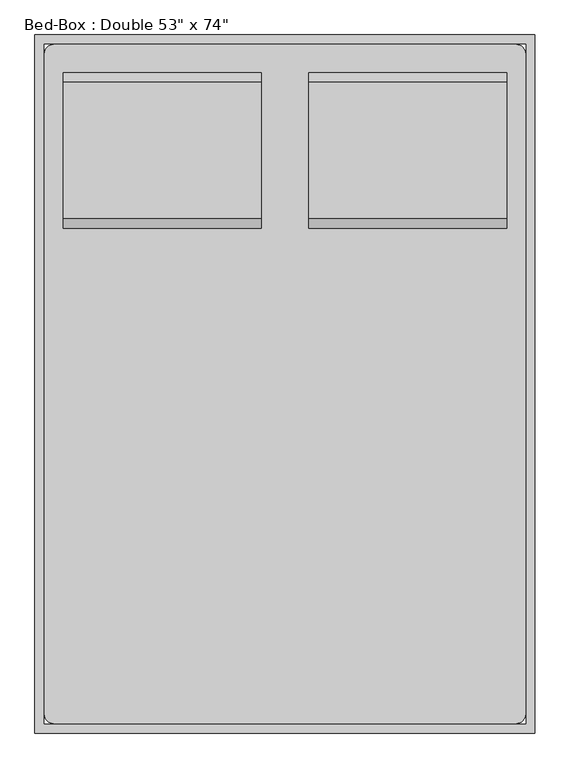
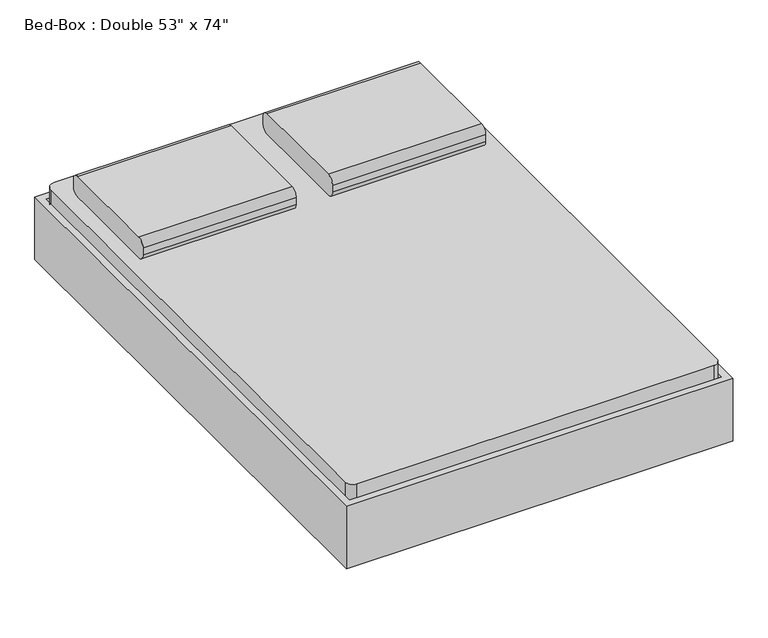
"""IFC4 building model written with IfcOpenShell, lengths in millimetres: furniture geometry."""

from ifc_helpers import new_model, si_unit, point, frame, frame_2d, origin, place, context, project, spatial, polyline, circle_curve, trimmed, segment, composite_curve, outline, extrude, source, transform, mapped, element, save
from ifc_brep_helpers import plane_surface, cylinder_surface, revolved_surface, advanced_brep


def furniture_c8abb964(model_context):
    return source(origin(), model_context, "Body", "SolidModel", [
        extrude(outline(composite_curve([segment(polyline([(578.3704918, 406.4), (210.0704918, 406.4)]), True, "CONTINUOUS"), segment(trimmed(circle_curve(frame_2d((210.0704918, 431.8)), 25.4), [point((210.0704918, 406.4))], [point((184.6704918, 431.8))], False, "CARTESIAN"), True, "CONTINUOUS"), segment(polyline([(184.6704918, 431.8), (184.6704918, 457.2)]), True, "CONTINUOUS"), segment(trimmed(circle_curve(frame_2d((210.0704918, 457.2)), 25.4), [point((184.6704918, 457.2))], [point((210.0704918, 482.6))], False, "CARTESIAN"), True, "CONTINUOUS"), segment(polyline([(210.0704918, 482.6), (578.3704918, 482.6)]), True, "CONTINUOUS"), segment(trimmed(circle_curve(frame_2d((578.3704918, 457.2)), 25.4), [point((578.3704918, 482.6))], [point((603.7704918, 457.2))], False, "CARTESIAN"), True, "CONTINUOUS"), segment(polyline([(603.7704918, 457.2), (603.7704918, 431.8)]), True, "CONTINUOUS"), segment(trimmed(circle_curve(frame_2d((578.3704918, 431.8)), 25.4), [point((603.7704918, 431.8))], [point((578.3704918, 406.4))], False, "CARTESIAN"), True, "CONTINUOUS")], self_intersect=False)), frame((402.652459, 0.0, 0.0), z_axis=(1.0, 0.0, 0.0), x_axis=(0.0, 1.0, 0.0)), (0.0, 0.0, 1.0), 533.4),
        extrude(outline(composite_curve([segment(polyline([(578.3704918, 406.4), (210.0704918, 406.4)]), True, "CONTINUOUS"), segment(trimmed(circle_curve(frame_2d((210.0704918, 431.8)), 25.4), [point((210.0704918, 406.4))], [point((184.6704918, 431.8))], False, "CARTESIAN"), True, "CONTINUOUS"), segment(polyline([(184.6704918, 431.8), (184.6704918, 457.2)]), True, "CONTINUOUS"), segment(trimmed(circle_curve(frame_2d((210.0704918, 457.2)), 25.4), [point((184.6704918, 457.2))], [point((210.0704918, 482.6))], False, "CARTESIAN"), True, "CONTINUOUS"), segment(polyline([(210.0704918, 482.6), (578.3704918, 482.6)]), True, "CONTINUOUS"), segment(trimmed(circle_curve(frame_2d((578.3704918, 457.2)), 25.4), [point((578.3704918, 482.6))], [point((603.7704918, 457.2))], False, "CARTESIAN"), True, "CONTINUOUS"), segment(polyline([(603.7704918, 457.2), (603.7704918, 431.8)]), True, "CONTINUOUS"), segment(trimmed(circle_curve(frame_2d((578.3704918, 431.8)), 25.4), [point((603.7704918, 431.8))], [point((578.3704918, 406.4))], False, "CARTESIAN"), True, "CONTINUOUS")], self_intersect=False)), frame((-257.747541, 0.0, 0.0), z_axis=(1.0, 0.0, 0.0), x_axis=(0.0, 1.0, 0.0)), (0.0, 0.0, 1.0), 533.4),
        advanced_brep(
        [(-308.2231784, 451.3704918, 177.8), (-308.2231784, 375.1704918, 177.8), (-308.2231784, 375.1704918, 196.85), (-308.2231784, 451.3704918, 196.85), (-257.4231784, 451.3704918, 177.8), (-257.4231784, 375.1704918, 177.8), (-245.2869899, 375.1704918, 196.85), (-245.2869899, 451.3704918, 196.85), (-181.3523099, 451.3704918, 14.6654962), (-181.3523099, 375.1704918, 14.6654962), (-164.0871466, 375.1704918, 22.716374), (-164.0871466, 451.3704918, 22.716374), (-158.3320921, 375.1704918, 0.0), (-158.3320921, 451.3704918, 0.0), (-158.3320921, 375.1704918, 19.05), (-158.3320921, 451.3704918, 19.05), (-79.7195862, 451.3704918, 0.0), (-79.7195862, 375.1704918, 0.0), (-79.7195862, 375.1704918, 19.05), (-79.7195862, 451.3704918, 19.05), (-67.0195862, 375.1704918, 3.4029547), (-67.0195862, 451.3704918, 3.4029547), (-76.5445862, 375.1704918, 19.9007387), (-76.5445862, 451.3704918, 19.9007387), (-6.922541, 451.3704918, 38.1), (-6.922541, 375.1704918, 38.1), (-12.0269731, 375.1704918, 57.15), (-12.0269731, 451.3704918, 57.15), (685.5518216, 451.3704918, 38.1), (685.5518216, 375.1704918, 38.1), (690.6562537, 375.1704918, 57.15), (690.6562537, 451.3704918, 57.15), (745.6488669, 451.3704918, 3.4029547), (745.6488669, 375.1704918, 3.4029547), (755.1738669, 375.1704918, 19.9007387), (755.1738669, 451.3704918, 19.9007387), (758.3488669, 375.1704918, 0.0), (758.3488669, 451.3704918, 0.0), (758.3488669, 375.1704918, 19.05), (758.3488669, 451.3704918, 19.05), (836.9613728, 451.3704918, 0.0), (836.9613728, 375.1704918, 0.0), (836.9613728, 375.1704918, 19.05), (836.9613728, 451.3704918, 19.05), (859.9815906, 375.1704918, 14.6654962), (859.9815906, 451.3704918, 14.6654962), (842.7164272, 375.1704918, 22.716374), (842.7164272, 451.3704918, 22.716374), (936.052459, 451.3704918, 177.8), (936.052459, 375.1704918, 177.8), (923.9162705, 375.1704918, 196.85), (923.9162705, 451.3704918, 196.85), (986.852459, 451.3704918, 177.8), (986.852459, 451.3704918, 196.85), (986.852459, 375.1704918, 196.85), (986.852459, 375.1704918, 177.8)],
        [
            (0, 1),
            (1, 2),
            (2, 3),
            (3, 0),
            (0, 4),
            (4, 5),
            (5, 1),
            (5, 6),
            (6, 2),
            (6, 7),
            (7, 3),
            (7, 4),
            (4, 8),
            (8, 9),
            (9, 5),
            (9, 10),
            (10, 6),
            (10, 11),
            (11, 7),
            (11, 8),
            (12, 9, circle_curve(frame((-158.3320921, 375.1704918, 25.4), z_axis=(0.0, 1.0, 0.0), x_axis=(-0.9063077870366486, 0.0, -0.42261826174070233)), 25.4)),
            (8, 13, circle_curve(frame((-158.3320921, 451.3704918, 25.4), z_axis=(0.0, -1.0, 0.0), x_axis=(-0.9063077870366486, 0.0, -0.42261826174070233)), 25.4)),
            (13, 12),
            (14, 10, circle_curve(frame((-158.3320921, 375.1704918, 25.4), z_axis=(0.0, 1.0, 0.0), x_axis=(-0.9063077870366486, 0.0, -0.42261826174070233)), 6.35)),
            (12, 14),
            (15, 11, circle_curve(frame((-158.3320921, 451.3704918, 25.4), z_axis=(0.0, 1.0, 0.0), x_axis=(-0.9063077870366486, 0.0, -0.42261826174070233)), 6.35)),
            (14, 15),
            (15, 13),
            (13, 16),
            (16, 17),
            (17, 12),
            (17, 18),
            (18, 14),
            (18, 19),
            (19, 15),
            (19, 16),
            (20, 17, circle_curve(frame((-79.7195862, 375.1704918, 25.4), z_axis=(0.0, 1.0, 0.0), x_axis=(0.0, 0.0, -1.0)), 25.4)),
            (16, 21, circle_curve(frame((-79.7195862, 451.3704918, 25.4), z_axis=(0.0, -1.0, 0.0), x_axis=(0.0, 0.0, -1.0)), 25.4)),
            (21, 20),
            (22, 18, circle_curve(frame((-79.7195862, 375.1704918, 25.4), z_axis=(0.0, 1.0, 0.0), x_axis=(0.0, 0.0, -1.0)), 6.35)),
            (20, 22),
            (23, 19, circle_curve(frame((-79.7195862, 451.3704918, 25.4), z_axis=(0.0, 1.0, 0.0), x_axis=(0.0, 0.0, -1.0)), 6.35)),
            (22, 23),
            (23, 21),
            (21, 24),
            (24, 25),
            (25, 20),
            (25, 26),
            (26, 22),
            (26, 27),
            (27, 23),
            (27, 24),
            (24, 28),
            (28, 29),
            (29, 25),
            (29, 30),
            (30, 26),
            (30, 31),
            (31, 27),
            (31, 28),
            (28, 32),
            (32, 33),
            (33, 29),
            (33, 34),
            (34, 30),
            (34, 35),
            (35, 31),
            (35, 32),
            (36, 33, circle_curve(frame((758.3488669, 375.1704918, 25.4), z_axis=(0.0, 1.0, 0.0), x_axis=(-0.5000000000000463, 0.0, -0.8660254037844118)), 25.4)),
            (32, 37, circle_curve(frame((758.3488669, 451.3704918, 25.4), z_axis=(0.0, -1.0, 0.0), x_axis=(-0.5000000000000463, 0.0, -0.8660254037844118)), 25.4)),
            (37, 36),
            (38, 34, circle_curve(frame((758.3488669, 375.1704918, 25.4), z_axis=(0.0, 1.0, 0.0), x_axis=(-0.5000000000000463, 0.0, -0.8660254037844118)), 6.35)),
            (36, 38),
            (39, 35, circle_curve(frame((758.3488669, 451.3704918, 25.4), z_axis=(0.0, 1.0, 0.0), x_axis=(-0.5000000000000463, 0.0, -0.8660254037844118)), 6.35)),
            (38, 39),
            (39, 37),
            (37, 40),
            (40, 41),
            (41, 36),
            (41, 42),
            (42, 38),
            (42, 43),
            (43, 39),
            (43, 40),
            (44, 41, circle_curve(frame((836.9613728, 375.1704918, 25.4), z_axis=(0.0, 1.0, 0.0), x_axis=(0.0, 0.0, -1.0)), 25.4)),
            (40, 45, circle_curve(frame((836.9613728, 451.3704918, 25.4), z_axis=(0.0, -1.0, 0.0), x_axis=(0.0, 0.0, -1.0)), 25.4)),
            (45, 44),
            (46, 42, circle_curve(frame((836.9613728, 375.1704918, 25.4), z_axis=(0.0, 1.0, 0.0), x_axis=(0.0, 0.0, -1.0)), 6.35)),
            (44, 46),
            (47, 43, circle_curve(frame((836.9613728, 451.3704918, 25.4), z_axis=(0.0, 1.0, 0.0), x_axis=(0.0, 0.0, -1.0)), 6.35)),
            (46, 47),
            (47, 45),
            (45, 48),
            (48, 49),
            (49, 44),
            (49, 50),
            (50, 46),
            (50, 51),
            (51, 47),
            (51, 48),
            (52, 53),
            (53, 54),
            (54, 55),
            (55, 52),
            (48, 52),
            (55, 49),
            (54, 50),
            (53, 51),
        ],
        [
            plane_surface(frame((-308.2231784, 705.3704918, -152.9490627), z_axis=(-1.0, 0.0, 0.0), x_axis=(0.0, 1.0, 0.0))),
            plane_surface(frame((-308.2231784, 451.3704918, 177.8), z_axis=(0.0, 0.0, -1.0), x_axis=(1.0, 0.0, 0.0))),
            plane_surface(frame((-308.2231784, 375.1704918, 177.8), z_axis=(0.0, -1.0, 0.0), x_axis=(1.0, 0.0, 0.0))),
            plane_surface(frame((-308.2231784, 375.1704918, 196.85), z_axis=(0.0, 0.0, 1.0), x_axis=(1.0, 0.0, 0.0))),
            plane_surface(frame((-308.2231784, 451.3704918, 196.85), z_axis=(0.0, 1.0, 0.0), x_axis=(1.0, 0.0, 0.0))),
            plane_surface(frame((-257.4231784, 451.3704918, 177.8), z_axis=(-0.9063077870366488, 0.0, -0.42261826174070194), x_axis=(0.42261826174070194, 0.0, -0.9063077870366488))),
            plane_surface(frame((-257.4231784, 375.1704918, 177.8), z_axis=(0.0, -1.0, 0.0), x_axis=(0.42261826174070194, 0.0, -0.9063077870366488))),
            plane_surface(frame((-245.2869899, 375.1704918, 196.85), z_axis=(0.9063077870366487, 0.0, 0.4226182617407021), x_axis=(0.4226182617407021, 0.0, -0.9063077870366487))),
            plane_surface(frame((-245.2869899, 451.3704918, 196.85), z_axis=(0.0, 1.0, 0.0), x_axis=(0.4226182617407021, 0.0, -0.9063077870366487))),
            cylinder_surface(frame((-158.3320921, 705.3704918, 25.4), z_axis=(0.0, -1.0, 0.0), x_axis=(-0.9063077870366486, 0.0, -0.42261826174070233)), 25.4),
            plane_surface(frame((-158.3320921, 375.1704918, 25.4), z_axis=(0.0, -1.0, 0.0), x_axis=(-0.9063077870366486, 0.0, -0.42261826174070233))),
            revolved_surface(polyline([(-164.08714654768272, 375.1704918, 22.71637403794654), (-164.08714654768272, 451.3704918, 22.71637403794654)]), (-158.3320921, 705.3704918, 25.4), (0.0, -1.0, 0.0)),
            plane_surface(frame((-158.3320921, 451.3704918, 25.4), z_axis=(0.0, 1.0, 0.0), x_axis=(-0.9063077870366486, 0.0, -0.42261826174070233))),
            plane_surface(frame((-158.3320921, 451.3704918, 0.0), z_axis=(0.0, 0.0, -1.0), x_axis=(1.0, 0.0, 0.0))),
            plane_surface(frame((-158.3320921, 375.1704918, 0.0), z_axis=(0.0, -1.0, 0.0), x_axis=(1.0, 0.0, 0.0))),
            plane_surface(frame((-158.3320921, 375.1704918, 19.05), z_axis=(0.0, 0.0, 1.0), x_axis=(1.0, 0.0, 0.0))),
            plane_surface(frame((-158.3320921, 451.3704918, 19.05), z_axis=(0.0, 1.0, 0.0), x_axis=(1.0, 0.0, 0.0))),
            cylinder_surface(frame((-79.7195862, 705.3704918, 25.4), z_axis=(0.0, -1.0, 0.0), x_axis=(0.0, 0.0, -1.0)), 25.4),
            plane_surface(frame((-79.7195862, 375.1704918, 25.4), z_axis=(0.0, -1.0, 0.0), x_axis=(0.0, 0.0, -1.0))),
            revolved_surface(polyline([(-79.7195862, 375.1704918, 19.049999999999997), (-79.7195862, 451.3704918, 19.049999999999997)]), (-79.7195862, 705.3704918, 25.4), (0.0, -1.0, 0.0)),
            plane_surface(frame((-79.7195862, 451.3704918, 25.4), z_axis=(0.0, 1.0, 0.0), x_axis=(0.0, 0.0, -1.0))),
            plane_surface(frame((-67.0195862, 451.3704918, 3.4029547), z_axis=(0.4999999999998775, 0.0, -0.8660254037845094), x_axis=(0.8660254037845094, 0.0, 0.4999999999998775))),
            plane_surface(frame((-67.0195862, 375.1704918, 3.4029547), z_axis=(0.0, -1.0, 0.0), x_axis=(0.866025403784509, 0.0, 0.49999999999987826))),
            plane_surface(frame((-76.5445862, 375.1704918, 19.9007387), z_axis=(-0.49999999999987754, 0.0, 0.8660254037845093), x_axis=(0.8660254037845093, 0.0, 0.49999999999987754))),
            plane_surface(frame((-76.5445862, 451.3704918, 19.9007387), z_axis=(0.0, 1.0000000000000002, 0.0), x_axis=(0.8660254037845091, 0.0, 0.49999999999987815))),
            plane_surface(frame((-6.922541, 451.3704918, 38.1), z_axis=(0.0, 0.0, -1.0), x_axis=(1.0, 0.0, 0.0))),
            plane_surface(frame((-6.922541, 375.1704918, 38.1), z_axis=(0.0, -1.0, 0.0), x_axis=(1.0, 0.0, 0.0))),
            plane_surface(frame((-12.0269731, 375.1704918, 57.15), z_axis=(0.0, 0.0, 1.0), x_axis=(1.0, 0.0, 0.0))),
            plane_surface(frame((-12.0269731, 451.3704918, 57.15), z_axis=(0.0, 1.0, 0.0), x_axis=(1.0, 0.0, 0.0))),
            plane_surface(frame((685.5518216, 451.3704918, 38.1), z_axis=(-0.500000000000047, 0.0, -0.8660254037844116), x_axis=(0.8660254037844116, 0.0, -0.500000000000047))),
            plane_surface(frame((685.5518216, 375.1704918, 38.1), z_axis=(0.0, -1.0, 0.0), x_axis=(0.8660254037844122, 0.0, -0.5000000000000459))),
            plane_surface(frame((690.6562537, 375.1704918, 57.15), z_axis=(0.5000000000000461, 0.0, 0.8660254037844121), x_axis=(0.8660254037844121, 0.0, -0.5000000000000461))),
            plane_surface(frame((690.6562537, 451.3704918, 57.15), z_axis=(0.0, 1.0, 0.0), x_axis=(0.8660254037844127, 0.0, -0.500000000000045))),
            cylinder_surface(frame((758.3488669, 705.3704918, 25.4), z_axis=(0.0, -1.0, 0.0), x_axis=(-0.5000000000000463, 0.0, -0.8660254037844118)), 25.4),
            plane_surface(frame((758.3488669, 375.1704918, 25.4), z_axis=(0.0, -1.0000000000000002, 0.0), x_axis=(-0.5000000000000464, 0.0, -0.866025403784412))),
            revolved_surface(polyline([(755.1738668999997, 375.1704918, 19.90073868596898), (755.1738668999997, 451.3704918, 19.90073868596898)]), (758.3488669, 705.3704918, 25.4), (0.0, -1.0, 0.0)),
            plane_surface(frame((758.3488669, 451.3704918, 25.4), z_axis=(0.0, 1.0000000000000002, 0.0), x_axis=(-0.5000000000000464, 0.0, -0.866025403784412))),
            plane_surface(frame((758.3488669, 451.3704918, 0.0), z_axis=(0.0, 0.0, -1.0), x_axis=(1.0, 0.0, 0.0))),
            plane_surface(frame((758.3488669, 375.1704918, 0.0), z_axis=(0.0, -1.0, 0.0), x_axis=(1.0, 0.0, 0.0))),
            plane_surface(frame((758.3488669, 375.1704918, 19.05), z_axis=(0.0, 0.0, 1.0), x_axis=(1.0, 0.0, 0.0))),
            plane_surface(frame((758.3488669, 451.3704918, 19.05), z_axis=(0.0, 1.0, 0.0), x_axis=(1.0, 0.0, 0.0))),
            cylinder_surface(frame((836.9613728, 705.3704918, 25.4), z_axis=(0.0, -1.0, 0.0), x_axis=(0.0, 0.0, -1.0)), 25.4),
            plane_surface(frame((836.9613728, 375.1704918, 25.4), z_axis=(0.0, -1.0, 0.0), x_axis=(0.0, 0.0, -1.0))),
            revolved_surface(polyline([(836.9613728, 375.1704918, 19.049999999999997), (836.9613728, 451.3704918, 19.049999999999997)]), (836.9613728, 705.3704918, 25.4), (0.0, -1.0, 0.0)),
            plane_surface(frame((836.9613728, 451.3704918, 25.4), z_axis=(0.0, 1.0, 0.0), x_axis=(0.0, 0.0, -1.0))),
            plane_surface(frame((859.9815906, 451.3704918, 14.6654962), z_axis=(0.9063077870366797, 0.0, -0.42261826174063566), x_axis=(0.42261826174063566, 0.0, 0.9063077870366797))),
            plane_surface(frame((859.9815906, 375.1704918, 14.6654962), z_axis=(0.0, -1.0000000000000002, 0.0), x_axis=(0.4226182617406349, 0.0, 0.9063077870366801))),
            plane_surface(frame((842.7164272, 375.1704918, 22.716374), z_axis=(-0.9063077870366799, 0.0, 0.4226182617406354), x_axis=(0.4226182617406354, 0.0, 0.9063077870366799))),
            plane_surface(frame((842.7164272, 451.3704918, 22.716374), z_axis=(0.0, 1.0, 0.0), x_axis=(0.42261826174063555, 0.0, 0.9063077870366798))),
            plane_surface(frame((986.852459, 705.3704918, -152.9490627), z_axis=(1.0, 0.0, 0.0), x_axis=(0.0, 1.0, 0.0))),
            plane_surface(frame((936.052459, 451.3704918, 177.8), z_axis=(0.0, 0.0, -1.0), x_axis=(1.0, 0.0, 0.0))),
            plane_surface(frame((936.052459, 375.1704918, 177.8), z_axis=(0.0, -1.0, 0.0), x_axis=(1.0, 0.0, 0.0))),
            plane_surface(frame((923.9162705, 375.1704918, 196.85), z_axis=(0.0, 0.0, 1.0), x_axis=(1.0, 0.0, 0.0))),
            plane_surface(frame((923.9162705, 451.3704918, 196.85), z_axis=(0.0, 1.0, 0.0), x_axis=(1.0, 0.0, 0.0))),
        ],
        [
            (0, [[1, 2, 3, 4]]),
            (1, [[-1, 5, 6, 7]]),
            (2, [[-2, -7, 8, 9]]),
            (3, [[-3, -9, 10, 11]]),
            (4, [[-4, -11, 12, -5]]),
            (5, [[-6, 13, 14, 15]]),
            (6, [[-8, -15, 16, 17]]),
            (7, [[-10, -17, 18, 19]]),
            (8, [[-12, -19, 20, -13]]),
            (9, [[21, -14, 22, 23]]),
            (10, [[24, -16, -21, 25]]),
            (11, [[26, -18, -24, 27]]),
            (12, [[-22, -20, -26, 28]]),
            (13, [[-23, 29, 30, 31]]),
            (14, [[-25, -31, 32, 33]]),
            (15, [[-27, -33, 34, 35]]),
            (16, [[-28, -35, 36, -29]]),
            (17, [[37, -30, 38, 39]]),
            (18, [[40, -32, -37, 41]]),
            (19, [[42, -34, -40, 43]]),
            (20, [[-38, -36, -42, 44]]),
            (21, [[-39, 45, 46, 47]]),
            (22, [[-41, -47, 48, 49]]),
            (23, [[-43, -49, 50, 51]]),
            (24, [[-44, -51, 52, -45]]),
            (25, [[-46, 53, 54, 55]]),
            (26, [[-48, -55, 56, 57]]),
            (27, [[-50, -57, 58, 59]]),
            (28, [[-52, -59, 60, -53]]),
            (29, [[-54, 61, 62, 63]]),
            (30, [[-56, -63, 64, 65]]),
            (31, [[-58, -65, 66, 67]]),
            (32, [[-60, -67, 68, -61]]),
            (33, [[69, -62, 70, 71]]),
            (34, [[72, -64, -69, 73]]),
            (35, [[74, -66, -72, 75]]),
            (36, [[-70, -68, -74, 76]]),
            (37, [[-71, 77, 78, 79]]),
            (38, [[-73, -79, 80, 81]]),
            (39, [[-75, -81, 82, 83]]),
            (40, [[-76, -83, 84, -77]]),
            (41, [[85, -78, 86, 87]]),
            (42, [[88, -80, -85, 89]]),
            (43, [[90, -82, -88, 91]]),
            (44, [[-86, -84, -90, 92]]),
            (45, [[-87, 93, 94, 95]]),
            (46, [[-89, -95, 96, 97]]),
            (47, [[-91, -97, 98, 99]]),
            (48, [[-92, -99, 100, -93]]),
            (49, [[101, 102, 103, 104]]),
            (50, [[-94, 105, -104, 106]]),
            (51, [[-96, -106, -103, 107]]),
            (52, [[-98, -107, -102, 108]]),
            (53, [[-100, -108, -101, -105]]),
        ],
    ),
        extrude(outline(composite_curve([segment(polyline([(-283.147541, 679.9704918), (961.452459, 679.9704918)]), True, "CONTINUOUS"), segment(trimmed(circle_curve(frame_2d((961.452459, 654.5704918)), 25.4), [point((961.452459, 679.9704918))], [point((986.852459, 654.5704918))], False, "CARTESIAN"), True, "CONTINUOUS"), segment(polyline([(986.852459, 654.5704918), (986.852459, -1123.4295082)]), True, "CONTINUOUS"), segment(trimmed(circle_curve(frame_2d((961.452459, -1123.4295082)), 25.4), [point((986.852459, -1123.4295082))], [point((961.452459, -1148.8295082))], False, "CARTESIAN"), True, "CONTINUOUS"), segment(polyline([(961.452459, -1148.8295082), (-283.147541, -1148.8295082)]), True, "CONTINUOUS"), segment(trimmed(circle_curve(frame_2d((-283.147541, -1123.4295082)), 25.4), [point((-283.147541, -1148.8295082))], [point((-308.547541, -1123.4295082))], False, "CARTESIAN"), True, "CONTINUOUS"), segment(polyline([(-308.547541, -1123.4295082), (-308.547541, 654.5704918)]), True, "CONTINUOUS"), segment(trimmed(circle_curve(frame_2d((-283.147541, 654.5704918)), 25.4), [point((-308.547541, 654.5704918))], [point((-283.147541, 679.9704918))], False, "CARTESIAN"), True, "CONTINUOUS")], self_intersect=False)), frame((0.0, 0.0, 203.2), z_axis=(0.0, 0.0, 1.0), x_axis=(1.0, 0.0, 0.0)), (0.0, 0.0, 1.0), 203.2),
        advanced_brep(
        [(-308.547541, -869.4295082, 196.85), (-308.547541, -869.4295082, 177.8), (-308.547541, -945.6295082, 177.8), (-308.547541, -945.6295082, 196.85), (-245.6113525, -869.4295082, 196.85), (-257.747541, -869.4295082, 177.8), (-257.747541, -945.6295082, 177.8), (-245.6113525, -945.6295082, 196.85), (-164.4115092, -869.4295082, 22.716374), (-181.6766725, -869.4295082, 14.6654962), (-181.6766725, -945.6295082, 14.6654962), (-164.4115092, -945.6295082, 22.716374), (-158.6564547, -869.4295082, 0.0), (-158.6564547, -869.4295082, 19.05), (-158.6564547, -945.6295082, 0.0), (-158.6564547, -945.6295082, 19.05), (-80.0439489, -869.4295082, 19.05), (-80.0439489, -869.4295082, 0.0), (-80.0439489, -945.6295082, 0.0), (-80.0439489, -945.6295082, 19.05), (-67.3439489, -869.4295082, 3.4029547), (-76.8689489, -869.4295082, 19.9007387), (-67.3439489, -945.6295082, 3.4029547), (-76.8689489, -945.6295082, 19.9007387), (-12.3513357, -869.4295082, 57.15), (-7.2469036, -869.4295082, 38.1), (-7.2469036, -945.6295082, 38.1), (-12.3513357, -945.6295082, 57.15), (690.6562537, -869.4295082, 57.15), (685.5518216, -869.4295082, 38.1), (685.5518216, -945.6295082, 38.1), (690.6562537, -945.6295082, 57.15), (755.1738669, -869.4295082, 19.9007387), (745.6488669, -869.4295082, 3.4029547), (745.6488669, -945.6295082, 3.4029547), (755.1738669, -945.6295082, 19.9007387), (758.3488669, -869.4295082, 0.0), (758.3488669, -869.4295082, 19.05), (758.3488669, -945.6295082, 0.0), (758.3488669, -945.6295082, 19.05), (836.9613728, -869.4295082, 19.05), (836.9613728, -869.4295082, 0.0), (836.9613728, -945.6295082, 0.0), (836.9613728, -945.6295082, 19.05), (859.9815906, -869.4295082, 14.6654962), (842.7164272, -869.4295082, 22.716374), (859.9815906, -945.6295082, 14.6654962), (842.7164272, -945.6295082, 22.716374), (923.9162705, -869.4295082, 196.85), (936.052459, -869.4295082, 177.8), (936.052459, -945.6295082, 177.8), (923.9162705, -945.6295082, 196.85), (986.852459, -869.4295082, 196.85), (986.852459, -945.6295082, 196.85), (986.852459, -945.6295082, 177.8), (986.852459, -869.4295082, 177.8)],
        [
            (0, 1),
            (1, 2),
            (2, 3),
            (3, 0),
            (0, 4),
            (4, 5),
            (5, 1),
            (5, 6),
            (6, 2),
            (6, 7),
            (7, 3),
            (7, 4),
            (4, 8),
            (8, 9),
            (9, 5),
            (9, 10),
            (10, 6),
            (10, 11),
            (11, 7),
            (11, 8),
            (12, 9, circle_curve(frame((-158.6564547, -869.4295082, 25.4), z_axis=(0.0, 1.0, 0.0), x_axis=(-0.906307787036663, 0.0, -0.4226182617406713)), 25.4)),
            (8, 13, circle_curve(frame((-158.6564547, -869.4295082, 25.4), z_axis=(0.0, -1.0, 0.0), x_axis=(-0.906307787036663, 0.0, -0.4226182617406713)), 6.35)),
            (13, 12),
            (14, 10, circle_curve(frame((-158.6564547, -945.6295082, 25.4), z_axis=(0.0, 1.0, 0.0), x_axis=(-0.906307787036663, 0.0, -0.4226182617406713)), 25.4)),
            (12, 14),
            (15, 11, circle_curve(frame((-158.6564547, -945.6295082, 25.4), z_axis=(0.0, 1.0, 0.0), x_axis=(-0.906307787036663, 0.0, -0.4226182617406713)), 6.35)),
            (14, 15),
            (15, 13),
            (13, 16),
            (16, 17),
            (17, 12),
            (17, 18),
            (18, 14),
            (18, 19),
            (19, 15),
            (19, 16),
            (20, 17, circle_curve(frame((-80.0439489, -869.4295082, 25.4), z_axis=(0.0, 1.0, 0.0), x_axis=(0.0, 0.0, -1.0)), 25.4)),
            (16, 21, circle_curve(frame((-80.0439489, -869.4295082, 25.4), z_axis=(0.0, -1.0, 0.0), x_axis=(0.0, 0.0, -1.0)), 6.35)),
            (21, 20),
            (22, 18, circle_curve(frame((-80.0439489, -945.6295082, 25.4), z_axis=(0.0, 1.0, 0.0), x_axis=(0.0, 0.0, -1.0)), 25.4)),
            (20, 22),
            (23, 19, circle_curve(frame((-80.0439489, -945.6295082, 25.4), z_axis=(0.0, 1.0, 0.0), x_axis=(0.0, 0.0, -1.0)), 6.35)),
            (22, 23),
            (23, 21),
            (21, 24),
            (24, 25),
            (25, 20),
            (25, 26),
            (26, 22),
            (26, 27),
            (27, 23),
            (27, 24),
            (24, 28),
            (28, 29),
            (29, 25),
            (29, 30),
            (30, 26),
            (30, 31),
            (31, 27),
            (31, 28),
            (28, 32),
            (32, 33),
            (33, 29),
            (33, 34),
            (34, 30),
            (34, 35),
            (35, 31),
            (35, 32),
            (36, 33, circle_curve(frame((758.3488669, -869.4295082, 25.4), z_axis=(0.0, 1.0, 0.0), x_axis=(-0.5000000000000479, 0.0, -0.866025403784411)), 25.4)),
            (32, 37, circle_curve(frame((758.3488669, -869.4295082, 25.4), z_axis=(0.0, -1.0, 0.0), x_axis=(-0.5000000000000479, 0.0, -0.866025403784411)), 6.35)),
            (37, 36),
            (38, 34, circle_curve(frame((758.3488669, -945.6295082, 25.4), z_axis=(0.0, 1.0, 0.0), x_axis=(-0.5000000000000479, 0.0, -0.866025403784411)), 25.4)),
            (36, 38),
            (39, 35, circle_curve(frame((758.3488669, -945.6295082, 25.4), z_axis=(0.0, 1.0, 0.0), x_axis=(-0.5000000000000479, 0.0, -0.866025403784411)), 6.35)),
            (38, 39),
            (39, 37),
            (37, 40),
            (40, 41),
            (41, 36),
            (41, 42),
            (42, 38),
            (42, 43),
            (43, 39),
            (43, 40),
            (44, 41, circle_curve(frame((836.9613728, -869.4295082, 25.4), z_axis=(0.0, 1.0, 0.0), x_axis=(0.0, 0.0, -1.0)), 25.4)),
            (40, 45, circle_curve(frame((836.9613728, -869.4295082, 25.4), z_axis=(0.0, -1.0, 0.0), x_axis=(0.0, 0.0, -1.0)), 6.35)),
            (45, 44),
            (46, 42, circle_curve(frame((836.9613728, -945.6295082, 25.4), z_axis=(0.0, 1.0, 0.0), x_axis=(0.0, 0.0, -1.0)), 25.4)),
            (44, 46),
            (47, 43, circle_curve(frame((836.9613728, -945.6295082, 25.4), z_axis=(0.0, 1.0, 0.0), x_axis=(0.0, 0.0, -1.0)), 6.35)),
            (46, 47),
            (47, 45),
            (45, 48),
            (48, 49),
            (49, 44),
            (49, 50),
            (50, 46),
            (50, 51),
            (51, 47),
            (51, 48),
            (52, 53),
            (53, 54),
            (54, 55),
            (55, 52),
            (48, 52),
            (55, 49),
            (54, 50),
            (53, 51),
        ],
        [
            plane_surface(frame((-308.547541, -1174.2295082, -127.5947323), z_axis=(-1.0, 0.0, 0.0), x_axis=(0.0, 1.0, 0.0))),
            plane_surface(frame((-308.547541, -869.4295082, 196.85), z_axis=(0.0, 1.0, 0.0), x_axis=(1.0, 0.0, 0.0))),
            plane_surface(frame((-308.547541, -869.4295082, 177.8), z_axis=(0.0, 0.0, -1.0), x_axis=(1.0, 0.0, 0.0))),
            plane_surface(frame((-308.547541, -945.6295082, 177.8), z_axis=(0.0, -1.0, 0.0), x_axis=(1.0, 0.0, 0.0))),
            plane_surface(frame((-308.547541, -945.6295082, 196.85), z_axis=(0.0, 0.0, 1.0), x_axis=(1.0, 0.0, 0.0))),
            plane_surface(frame((-245.6113525, -869.4295082, 196.85), z_axis=(0.0, 1.0, 0.0), x_axis=(0.422618261740671, 0.0, -0.9063077870366633))),
            plane_surface(frame((-257.747541, -869.4295082, 177.8), z_axis=(-0.9063077870366631, 0.0, -0.42261826174067113), x_axis=(0.42261826174067113, 0.0, -0.9063077870366631))),
            plane_surface(frame((-257.747541, -945.6295082, 177.8), z_axis=(0.0, -1.0, 0.0), x_axis=(0.42261826174067135, 0.0, -0.906307787036663))),
            plane_surface(frame((-245.6113525, -945.6295082, 196.85), z_axis=(0.9063077870366631, 0.0, 0.4226182617406713), x_axis=(0.4226182617406713, 0.0, -0.9063077870366631))),
            plane_surface(frame((-158.6564547, -869.4295082, 25.4), z_axis=(0.0, 1.0, 0.0), x_axis=(-0.906307787036663, 0.0, -0.4226182617406713))),
            cylinder_surface(frame((-158.6564547, -1174.2295082, 25.4), z_axis=(0.0, -1.0, 0.0), x_axis=(-0.906307787036663, 0.0, -0.4226182617406713)), 25.4),
            plane_surface(frame((-158.6564547, -945.6295082, 25.4), z_axis=(0.0, -1.0, 0.0), x_axis=(-0.906307787036663, 0.0, -0.4226182617406713))),
            revolved_surface(polyline([(-164.41150914768284, -945.6295082, 22.716374037946736), (-164.41150914768284, -869.4295082, 22.716374037946736)]), (-158.6564547, -1174.2295082, 25.4), (0.0, -1.0, 0.0)),
            plane_surface(frame((-158.6564547, -869.4295082, 19.05), z_axis=(0.0, 1.0, 0.0), x_axis=(1.0, 0.0, 0.0))),
            plane_surface(frame((-158.6564547, -869.4295082, 0.0), z_axis=(0.0, 0.0, -1.0), x_axis=(1.0, 0.0, 0.0))),
            plane_surface(frame((-158.6564547, -945.6295082, 0.0), z_axis=(0.0, -1.0, 0.0), x_axis=(1.0, 0.0, 0.0))),
            plane_surface(frame((-158.6564547, -945.6295082, 19.05), z_axis=(0.0, 0.0, 1.0), x_axis=(1.0, 0.0, 0.0))),
            plane_surface(frame((-80.0439489, -869.4295082, 25.4), z_axis=(0.0, 1.0, 0.0), x_axis=(0.0, 0.0, -1.0))),
            cylinder_surface(frame((-80.0439489, -1174.2295082, 25.4), z_axis=(0.0, -1.0, 0.0), x_axis=(0.0, 0.0, -1.0)), 25.4),
            plane_surface(frame((-80.0439489, -945.6295082, 25.4), z_axis=(0.0, -1.0, 0.0), x_axis=(0.0, 0.0, -1.0))),
            revolved_surface(polyline([(-80.0439489, -945.6295082, 19.049999999999997), (-80.0439489, -869.4295082, 19.049999999999997)]), (-80.0439489, -1174.2295082, 25.4), (0.0, -1.0, 0.0)),
            plane_surface(frame((-76.8689489, -869.4295082, 19.9007387), z_axis=(0.0, 1.0, 0.0), x_axis=(0.8660254037844785, 0.0, 0.499999999999931))),
            plane_surface(frame((-67.3439489, -869.4295082, 3.4029547), z_axis=(0.499999999999931, 0.0, -0.8660254037844785), x_axis=(0.8660254037844785, 0.0, 0.499999999999931))),
            plane_surface(frame((-67.3439489, -945.6295082, 3.4029547), z_axis=(0.0, -1.0, 0.0), x_axis=(0.8660254037844786, 0.0, 0.49999999999993094))),
            plane_surface(frame((-76.8689489, -945.6295082, 19.9007387), z_axis=(-0.4999999999999312, 0.0, 0.8660254037844785), x_axis=(0.8660254037844785, 0.0, 0.4999999999999312))),
            plane_surface(frame((-12.3513357, -869.4295082, 57.15), z_axis=(0.0, 1.0, 0.0), x_axis=(1.0, 0.0, 0.0))),
            plane_surface(frame((-7.2469036, -869.4295082, 38.1), z_axis=(0.0, 0.0, -1.0), x_axis=(1.0, 0.0, 0.0))),
            plane_surface(frame((-7.2469036, -945.6295082, 38.1), z_axis=(0.0, -1.0, 0.0), x_axis=(1.0, 0.0, 0.0))),
            plane_surface(frame((-12.3513357, -945.6295082, 57.15), z_axis=(0.0, 0.0, 1.0), x_axis=(1.0, 0.0, 0.0))),
            plane_surface(frame((690.6562537, -869.4295082, 57.15), z_axis=(0.0, 1.0, 0.0), x_axis=(0.8660254037844091, 0.0, -0.5000000000000514))),
            plane_surface(frame((685.5518216, -869.4295082, 38.1), z_axis=(-0.5000000000000502, 0.0, -0.8660254037844097), x_axis=(0.8660254037844097, 0.0, -0.5000000000000502))),
            plane_surface(frame((685.5518216, -945.6295082, 38.1), z_axis=(0.0, -1.0, 0.0), x_axis=(0.86602540378441, 0.0, -0.5000000000000498))),
            plane_surface(frame((690.6562537, -945.6295082, 57.15), z_axis=(0.5000000000000505, 0.0, 0.8660254037844095), x_axis=(0.8660254037844095, 0.0, -0.5000000000000505))),
            plane_surface(frame((758.3488669, -869.4295082, 25.4), z_axis=(0.0, 1.0000000000000002, 0.0), x_axis=(-0.500000000000048, 0.0, -0.8660254037844111))),
            cylinder_surface(frame((758.3488669, -1174.2295082, 25.4), z_axis=(0.0, -1.0, 0.0), x_axis=(-0.5000000000000479, 0.0, -0.866025403784411)), 25.4),
            plane_surface(frame((758.3488669, -945.6295082, 25.4), z_axis=(0.0, -1.0000000000000002, 0.0), x_axis=(-0.500000000000048, 0.0, -0.8660254037844111))),
            revolved_surface(polyline([(755.1738668999997, -945.6295082, 19.90073868596899), (755.1738668999997, -869.4295082, 19.90073868596899)]), (758.3488669, -1174.2295082, 25.4), (0.0, -1.0, 0.0)),
            plane_surface(frame((758.3488669, -869.4295082, 19.05), z_axis=(0.0, 1.0, 0.0), x_axis=(1.0, 0.0, 0.0))),
            plane_surface(frame((758.3488669, -869.4295082, 0.0), z_axis=(0.0, 0.0, -1.0), x_axis=(1.0, 0.0, 0.0))),
            plane_surface(frame((758.3488669, -945.6295082, 0.0), z_axis=(0.0, -1.0, 0.0), x_axis=(1.0, 0.0, 0.0))),
            plane_surface(frame((758.3488669, -945.6295082, 19.05), z_axis=(0.0, 0.0, 1.0), x_axis=(1.0, 0.0, 0.0))),
            plane_surface(frame((836.9613728, -869.4295082, 25.4), z_axis=(0.0, 1.0, 0.0), x_axis=(0.0, 0.0, -1.0))),
            cylinder_surface(frame((836.9613728, -1174.2295082, 25.4), z_axis=(0.0, -1.0, 0.0), x_axis=(0.0, 0.0, -1.0)), 25.4),
            plane_surface(frame((836.9613728, -945.6295082, 25.4), z_axis=(0.0, -1.0, 0.0), x_axis=(0.0, 0.0, -1.0))),
            revolved_surface(polyline([(836.9613728, -945.6295082, 19.049999999999997), (836.9613728, -869.4295082, 19.049999999999997)]), (836.9613728, -1174.2295082, 25.4), (0.0, -1.0, 0.0)),
            plane_surface(frame((842.7164272, -869.4295082, 22.716374), z_axis=(0.0, 1.0, 0.0), x_axis=(0.4226182617405411, 0.0, 0.9063077870367238))),
            plane_surface(frame((859.9815906, -869.4295082, 14.6654962), z_axis=(0.9063077870367237, 0.0, -0.42261826174054157), x_axis=(0.42261826174054157, 0.0, 0.9063077870367237))),
            plane_surface(frame((859.9815906, -945.6295082, 14.6654962), z_axis=(0.0, -1.0, 0.0), x_axis=(0.4226182617405412, 0.0, 0.9063077870367238))),
            plane_surface(frame((842.7164272, -945.6295082, 22.716374), z_axis=(-0.906307787036724, 0.0, 0.422618261740541), x_axis=(0.422618261740541, 0.0, 0.906307787036724))),
            plane_surface(frame((986.852459, -1174.2295082, -127.5947323), z_axis=(1.0, 0.0, 0.0), x_axis=(0.0, 1.0, 0.0))),
            plane_surface(frame((923.9162705, -869.4295082, 196.85), z_axis=(0.0, 1.0, 0.0), x_axis=(1.0, 0.0, 0.0))),
            plane_surface(frame((936.052459, -869.4295082, 177.8), z_axis=(0.0, 0.0, -1.0), x_axis=(1.0, 0.0, 0.0))),
            plane_surface(frame((936.052459, -945.6295082, 177.8), z_axis=(0.0, -1.0, 0.0), x_axis=(1.0, 0.0, 0.0))),
            plane_surface(frame((923.9162705, -945.6295082, 196.85), z_axis=(0.0, 0.0, 1.0), x_axis=(1.0, 0.0, 0.0))),
        ],
        [
            (0, [[1, 2, 3, 4]]),
            (1, [[-1, 5, 6, 7]]),
            (2, [[-2, -7, 8, 9]]),
            (3, [[-3, -9, 10, 11]]),
            (4, [[-4, -11, 12, -5]]),
            (5, [[-6, 13, 14, 15]]),
            (6, [[-8, -15, 16, 17]]),
            (7, [[-10, -17, 18, 19]]),
            (8, [[-12, -19, 20, -13]]),
            (9, [[21, -14, 22, 23]]),
            (10, [[24, -16, -21, 25]]),
            (11, [[26, -18, -24, 27]]),
            (12, [[-22, -20, -26, 28]]),
            (13, [[-23, 29, 30, 31]]),
            (14, [[-25, -31, 32, 33]]),
            (15, [[-27, -33, 34, 35]]),
            (16, [[-28, -35, 36, -29]]),
            (17, [[37, -30, 38, 39]]),
            (18, [[40, -32, -37, 41]]),
            (19, [[42, -34, -40, 43]]),
            (20, [[-38, -36, -42, 44]]),
            (21, [[-39, 45, 46, 47]]),
            (22, [[-41, -47, 48, 49]]),
            (23, [[-43, -49, 50, 51]]),
            (24, [[-44, -51, 52, -45]]),
            (25, [[-46, 53, 54, 55]]),
            (26, [[-48, -55, 56, 57]]),
            (27, [[-50, -57, 58, 59]]),
            (28, [[-52, -59, 60, -53]]),
            (29, [[-54, 61, 62, 63]]),
            (30, [[-56, -63, 64, 65]]),
            (31, [[-58, -65, 66, 67]]),
            (32, [[-60, -67, 68, -61]]),
            (33, [[69, -62, 70, 71]]),
            (34, [[72, -64, -69, 73]]),
            (35, [[74, -66, -72, 75]]),
            (36, [[-70, -68, -74, 76]]),
            (37, [[-71, 77, 78, 79]]),
            (38, [[-73, -79, 80, 81]]),
            (39, [[-75, -81, 82, 83]]),
            (40, [[-76, -83, 84, -77]]),
            (41, [[85, -78, 86, 87]]),
            (42, [[88, -80, -85, 89]]),
            (43, [[90, -82, -88, 91]]),
            (44, [[-86, -84, -90, 92]]),
            (45, [[-87, 93, 94, 95]]),
            (46, [[-89, -95, 96, 97]]),
            (47, [[-91, -97, 98, 99]]),
            (48, [[-92, -99, 100, -93]]),
            (49, [[101, 102, 103, 104]]),
            (50, [[-94, 105, -104, 106]]),
            (51, [[-96, -106, -103, 107]]),
            (52, [[-98, -107, -102, 108]]),
            (53, [[-100, -108, -101, -105]]),
        ],
    ),
        extrude(outline(polyline([(1012.252459, 705.3704918), (1012.252459, -1174.2295082), (-333.947541, -1174.2295082), (-333.947541, 705.3704918), (1012.252459, 705.3704918)]), holes=[polyline([(986.852459, 679.9704918), (-308.547541, 679.9704918), (-308.547541, -1148.8295082), (986.852459, -1148.8295082), (986.852459, 679.9704918)])]), frame((0.0, 0.0, 127.0), z_axis=(0.0, 0.0, 1.0), x_axis=(1.0, 0.0, 0.0)), (0.0, 0.0, 1.0), 228.6),
    ])


if __name__ == "__main__":
    model = new_model("IFC4")
    model_context = context("Model", 3, world=origin())
    ifc_project = project(units=[si_unit("LENGTHUNIT", "METRE", prefix="MILLI")], contexts=[model_context])
    site = spatial("IfcSite", under=ifc_project)
    building = spatial("IfcBuilding", under=site)
    placement = place(None, origin())
    furniture_shape = furniture_c8abb964(model_context)
    element("IfcFurniture", 1, ObjectType="Bed-Box : Double 53\" x 74\"", at=placement, inside=building, context=model_context, shape_type="MappedRepresentation", body=[
        mapped(furniture_shape, transform((0.0, 0.0, 0.0), x_axis=(1.0, 0.0, 0.0), y_axis=(0.0, 1.0, 0.0), z_axis=(0.0, 0.0, 1.0))),
    ])
    save(model, "model.ifc")

# Revit data of these elements
# Type "Bed-Box : Double 53\" x 74\""
#   Assembly Code = "E2020200"
#   Length = 6' - 2"
#   Width = 4' - 5"
#   Frame Material = Birch
#   Mattress Material = Cherry
#   Default Elevation = 0
# Element 1 (IfcFurniture, "Bed-Box : Double 53\" x 74\"")
#   Materials on its faces: "Birch", "Cherry"
# Materials
#   "Birch": class "Wood", colour RGB 224 178 126, transparency 0, Description = "Betula Alleghaniensis", Cost = 0
#   "Cherry": class "Wood", colour RGB 226 177 128, transparency 0, Description = "Prunus Serotina", Cost = 0
